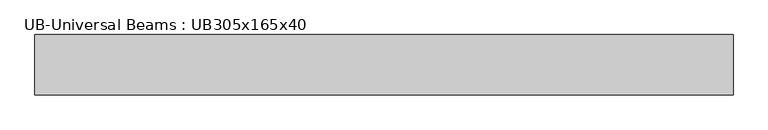
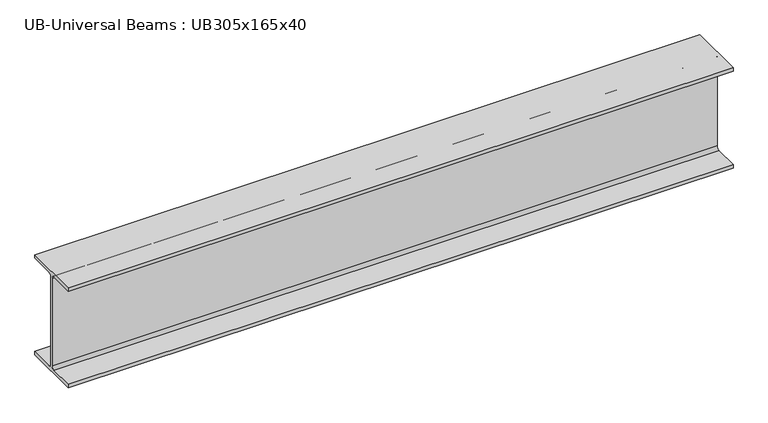
"""IFC4 building model written with IfcOpenShell, lengths in millimetres: beam geometry, UB-Universal Beams : UB305x165x40."""

from ifc_helpers import new_model, si_unit, point, frame, frame_2d, origin, place, context, project, spatial, polyline, circle_curve, trimmed, segment, composite_curve, outline, extrude, source, transform, mapped, element, save


def ub_universal_beams_ub305x165x40_46279f85(model_context):
    return source(origin(), model_context, "Body", "SweptSolid", [
        extrude(outline(composite_curve([segment(polyline([(82.5, -141.5), (82.5, -151.7), (-82.5, -151.7), (-82.5, -141.5), (-11.9, -141.5)]), True, "CONTINUOUS"), segment(trimmed(circle_curve(frame_2d((-11.9, -132.6)), 8.9), [point((-11.9, -141.5))], [point((-3.0, -132.6))], True, "CARTESIAN"), True, "CONTINUOUS"), segment(polyline([(-3.0, -132.6), (-3.0, 132.6)]), True, "CONTINUOUS"), segment(trimmed(circle_curve(frame_2d((-11.9, 132.6)), 8.9), [point((-3.0, 132.6))], [point((-11.9, 141.5))], True, "CARTESIAN"), True, "CONTINUOUS"), segment(polyline([(-11.9, 141.5), (-82.5, 141.5), (-82.5, 151.7), (82.5, 151.7), (82.5, 141.5), (11.9, 141.5)]), True, "CONTINUOUS"), segment(trimmed(circle_curve(frame_2d((11.9, 132.6)), 8.9), [point((11.9, 141.5))], [point((3.0, 132.6))], True, "CARTESIAN"), True, "CONTINUOUS"), segment(polyline([(3.0, 132.6), (3.0, -132.6)]), True, "CONTINUOUS"), segment(trimmed(circle_curve(frame_2d((11.9, -132.6)), 8.9), [point((3.0, -132.6))], [point((11.9, -141.5))], True, "CARTESIAN"), True, "CONTINUOUS"), segment(polyline([(11.9, -141.5), (82.5, -141.5)]), True, "CONTINUOUS")], self_intersect=False)), frame((-1069.95, 0.0, 0.0), z_axis=(1.0, 0.0, 0.0), x_axis=(0.0, 1.0, 0.0)), (0.0, 0.0, 1.0), 1905.0),
    ])


if __name__ == "__main__":
    model = new_model("IFC4")
    model_context = context("Model", 3, world=origin())
    ifc_project = project(units=[si_unit("LENGTHUNIT", "METRE", prefix="MILLI")], contexts=[model_context])
    site = spatial("IfcSite", under=ifc_project)
    building = spatial("IfcBuilding", under=site)
    placement = place(None, origin())
    ub_universal_beams_ub305x165x40_shape = ub_universal_beams_ub305x165x40_46279f85(model_context)
    element("IfcBeam", 1, ObjectType="UB-Universal Beams : UB305x165x40", at=placement, inside=building, context=model_context, shape_type="MappedRepresentation", body=[
        mapped(ub_universal_beams_ub305x165x40_shape, transform((0.0, 0.0, 0.0), x_axis=(1.0, 0.0, 0.0), y_axis=(0.0, 1.0, 0.0), z_axis=(0.0, 0.0, 1.0))),
    ])
    save(model, "model.ifc")

# Revit data of these elements
# Type "UB-Universal Beams : UB305x165x40"
#   Section Name Key = "UB305X165X40"
#   Width = 16.5 cm
#   Web Thickness = 0.6 cm
#   Web Fillet = 0.89 cm
#   Warping Constant = 164000.0 cm⁶
#   Torsional Moment of Inertia = 14.70 cm⁴
#   Section Area = 51.3 cm²
#   Plastic Modulus weak axis = 142.0 cm³
#   Plastic Modulus strong axis = 623.0 cm³
#   Nominal Weight = 40.2999 kgf/m
#   Moment of Inertia weak axis = 764.00 cm⁴
#   Moment of Inertia strong axis = 8503.00 cm⁴
#   Height = 30.34 cm
#   Flange Thickness = 1.02 cm
#   Elastic Modulus weak axis = 92.6 cm³
#   Elastic Modulus strong axis = 560.0 cm³
#   Centroid Vertical = 15.17 cm
#   Centroid Horizontal = 8.25 cm
#   Bolt Spacing = 9.0 cm
#   Length [instance default] = 1500 mm
#   Structural Material [instance default] = Metal - Steel 43-275
#   Type Comments = ""
#   Assembly Code = ""
# Element 1 (IfcBeam, "UB-Universal Beams : UB305x165x40")
#   Materials on its faces: "Metal - Steel 43-275"
# Materials
#   "Metal - Steel 43-275": class "Metal", colour RGB 247 247 247, transparency 0, Cost = 0
